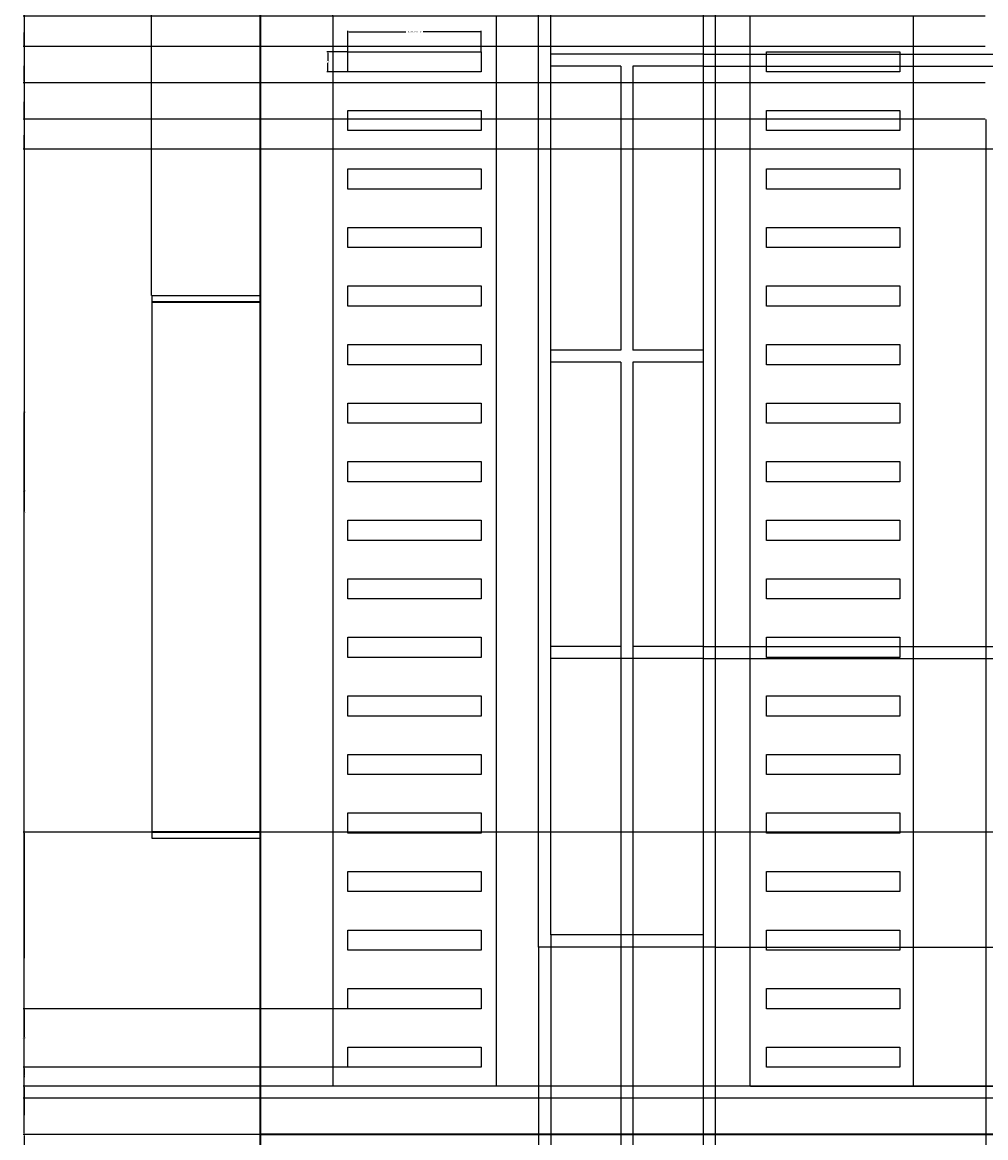
# Model space of a CAD drawing. Units: inches. Extents: x 2148 to 2587, y 1015 to 1466.
# Tile 4 of 7: x 2148 to 2307, y 1166 to 1351. Entities that reach past the tile are written whole.
import ezdxf

# ---------------------------------------------------------------- set-up
doc = ezdxf.new("R2010")
doc.units = ezdxf.units.IN
for name, color, linetype, lineweight in [('A-ANNO-DIMS', 2, 'Continuous', 18), ('A-ELEV', 7, 'Continuous', 35), ('A-GLAZ', 4, 'Continuous', 25)]:
    doc.layers.add(name, color=color, linetype=linetype, lineweight=lineweight)
doc.styles.get("Standard").update_dxf_attribs({"font": 'arial.ttf'})
doc.dimstyles.get("Standard").update_dxf_attribs({"dimtxt": 0.18, "dimasz": 0.18, "dimexe": 0.18, "dimexo": 0.0625, "dimgap": 0.09, "dimtad": 0, "dimtih": 1, "dimtoh": 1, "dimdec": 4, "dimzin": 0, "dimdsep": 46, "dimtxsty": 'Standard', "dimcen": 0.09, "dimadec": 0, "dimazin": 0, "dimtfac": 1, "dimtdec": 4, "dimtofl": 0, "dimtmove": 0, "dimatfit": 3, "dimfxl": 1, "dimtolj": 1, "dimtzin": 0, "dimarcsym": 0})

# ---------------------------------------------------------------- blocks, each defined once
blk = doc.blocks.new('WIN-SIDE')
for p, q in [((18, 89.73), (0, 89.73)), ((18, 0), (18, 89.73)), ((0, 0), (18, 0))]:
    blk.add_line(p, q)
blk = doc.blocks.new('LOUVRE-SLAT')
blk.add_lwpolyline([(2201.49, 1345.86), (2223.57, 1345.86), (2223.57, 1342.52), (2201.49, 1342.52)], close=True)
blk = doc.blocks.new('*D3')
at = {"layer": 'A-ANNO-DIMS', "color": 0, "lineweight": -2, "transparency": 16777216}
for p, q in [((2201.49, 1345.92), (2201.49, 1349.35)), ((2201.67, 1349.17), (2211.11, 1349.17)), ((2223.39, 1349.17), (2213.96, 1349.17)), ((2223.57, 1345.92), (2223.57, 1349.35))]:
    blk.add_line(p, q, dxfattribs=at)
at = {"layer": 'A-ANNO-DIMS', "color": 0, "transparency": 16777216}
for points in [[(2201.67, 1349.2), (2201.67, 1349.14), (2201.49, 1349.17)], [(2223.39, 1349.2), (2223.39, 1349.14), (2223.57, 1349.17)]]:
    blk.add_solid(points, dxfattribs=at)
at = {"layer": 'Defpoints', "color": 0, "transparency": 16777216}
for p in [(2223.57, 1349.17), (2201.49, 1345.86), (2223.57, 1345.86)]:
    blk.add_point(p, dxfattribs=at)
at = {"layer": 'A-ANNO-DIMS', "color": 0, "transparency": 16777216, "insert": (2212.53, 1349.17), "char_height": 0.18, "attachment_point": 5}
blk.add_mtext('\\A1;LOUVRE SLAT 22 TYP.', dxfattribs=at)
blk = doc.blocks.new('*D4')
at = {"layer": 'A-ANNO-DIMS', "color": 0, "lineweight": -2, "transparency": 16777216}
for p, q in [((2201.43, 1345.86), (2198, 1345.86)), ((2198.18, 1345.68), (2198.18, 1344.37)), ((2198.18, 1342.7), (2198.18, 1344.01)), ((2201.43, 1342.52), (2198, 1342.52))]:
    blk.add_line(p, q, dxfattribs=at)
at = {"layer": 'A-ANNO-DIMS', "color": 0, "transparency": 16777216}
for points in [[(2198.15, 1345.68), (2198.21, 1345.68), (2198.18, 1345.86)], [(2198.15, 1342.7), (2198.21, 1342.7), (2198.18, 1342.52)]]:
    blk.add_solid(points, dxfattribs=at)
at = {"layer": 'Defpoints', "color": 0, "transparency": 16777216}
for p in [(2198.18, 1345.86), (2201.49, 1345.86), (2201.49, 1342.52)]:
    blk.add_point(p, dxfattribs=at)
at = {"layer": 'A-ANNO-DIMS', "color": 0, "transparency": 16777216, "insert": (2198.18, 1344.19), "char_height": 0.18, "attachment_point": 5}
blk.add_mtext('\\A1;3 TYP.', dxfattribs=at)
blk = doc.blocks.new('*D7')
at = {"layer": 'A-ANNO-DIMS', "color": 0, "lineweight": -2, "transparency": 16777216}
for p, q in [((2169.03, 1305.54), (2169.03, 1466.02)), ((2169.21, 1465.84), (2175.82, 1465.84)), ((2182.85, 1465.84), (2176.24, 1465.84)), ((2183.03, 1444.81), (2183.03, 1466.02))]:
    blk.add_line(p, q, dxfattribs=at)
at = {"layer": 'A-ANNO-DIMS', "color": 0, "transparency": 16777216}
for points in [[(2169.21, 1465.87), (2169.21, 1465.81), (2169.03, 1465.84)], [(2182.85, 1465.87), (2182.85, 1465.81), (2183.03, 1465.84)]]:
    blk.add_solid(points, dxfattribs=at)
at = {"layer": 'Defpoints', "color": 0, "transparency": 16777216}
for p in [(2183.03, 1465.84), (2183.03, 1444.74), (2169.03, 1305.47)]:
    blk.add_point(p, dxfattribs=at)
at = {"layer": 'A-ANNO-DIMS', "color": 0, "transparency": 16777216, "insert": (2176.03, 1465.84), "char_height": 0.18, "attachment_point": 5}
blk.add_mtext('\\A1;14', dxfattribs=at)
blk = doc.blocks.new('*D22')
at = {"layer": 'A-ANNO-DIMS', "color": 0, "lineweight": -2, "transparency": 16777216}
for p, q in [((2186.971769, 1166.74266), (2147.754269, 1166.74266)), ((2147.934269, 1166.56266), (2147.934269, 1164.92266)), ((2147.934269, 1162.92266), (2147.934269, 1164.56266)), ((2186.971769, 1162.74266), (2147.754269, 1162.74266))]:
    blk.add_line(p, q, dxfattribs=at)
at = {"layer": 'A-ANNO-DIMS', "color": 0, "transparency": 16777216}
for points in [[(2147.904269, 1166.56266), (2147.964269, 1166.56266), (2147.934269, 1166.74266)], [(2147.904269, 1162.92266), (2147.964269, 1162.92266), (2147.934269, 1162.74266)]]:
    blk.add_solid(points, dxfattribs=at)
at = {"layer": 'Defpoints', "color": 0, "transparency": 16777216}
for p in [(2147.934269, 1166.74266), (2187.034269, 1166.74266), (2187.034269, 1162.74266)]:
    blk.add_point(p, dxfattribs=at)
at = {"layer": 'A-ANNO-DIMS', "color": 0, "transparency": 16777216, "insert": (2147.934269, 1164.74266), "char_height": 0.18, "attachment_point": 5}
blk.add_mtext('\\A1;4', dxfattribs=at)
blk = doc.blocks.new('*D23')
at = {"layer": 'A-ANNO-DIMS', "color": 0, "lineweight": -2, "transparency": 16777216}
for p, q in [((2186.97, 1405.74), (2147.75, 1405.74)), ((2147.93, 1405.56), (2147.93, 1286.42)), ((2147.93, 1166.92), (2147.93, 1286.06)), ((2186.97, 1166.74), (2147.75, 1166.74))]:
    blk.add_line(p, q, dxfattribs=at)
at = {"layer": 'A-ANNO-DIMS', "color": 0, "transparency": 16777216}
for points in [[(2147.9, 1405.56), (2147.96, 1405.56), (2147.93, 1405.74)], [(2147.9, 1166.92), (2147.96, 1166.92), (2147.93, 1166.74)]]:
    blk.add_solid(points, dxfattribs=at)
at = {"layer": 'Defpoints', "color": 0, "transparency": 16777216}
for p in [(2147.93, 1405.74), (2187.03, 1405.74), (2187.03, 1166.74)]:
    blk.add_point(p, dxfattribs=at)
at = {"layer": 'A-ANNO-DIMS', "color": 0, "transparency": 16777216, "insert": (2147.93, 1286.24), "char_height": 0.18, "attachment_point": 5}
blk.add_mtext('\\A1;239', dxfattribs=at)
blk = doc.blocks.new('*D47')
at = {"layer": 'A-ANNO-DIMS', "color": 0, "lineweight": -2, "transparency": 16777216}
for p, q in [((2307.03, 1334.68), (2307.03, 1015.46)), ((2316.03, 1329.68), (2316.03, 1015.46)), ((2307.21, 1015.64), (2311.39, 1015.64)), ((2315.85, 1015.64), (2311.68, 1015.64))]:
    blk.add_line(p, q, dxfattribs=at)
at = {"layer": 'A-ANNO-DIMS', "color": 0, "transparency": 16777216}
for points in [[(2307.21, 1015.67), (2307.21, 1015.61), (2307.03, 1015.64)], [(2315.85, 1015.67), (2315.85, 1015.61), (2316.03, 1015.64)]]:
    blk.add_solid(points, dxfattribs=at)
at = {"layer": 'Defpoints', "color": 0, "transparency": 16777216}
for p in [(2307.03, 1334.74), (2316.03, 1329.74), (2316.03, 1015.64)]:
    blk.add_point(p, dxfattribs=at)
at = {"layer": 'A-ANNO-DIMS', "color": 0, "transparency": 16777216, "insert": (2311.53, 1015.64), "char_height": 0.18, "attachment_point": 5}
blk.add_mtext('\\A1;9', dxfattribs=at)
blk = doc.blocks.new('*D58')
at = {"layer": 'A-ANNO-DIMS', "color": 0, "lineweight": -2, "transparency": 16777216}
for p, q in [((2306.971769, 1166.74266), (2147.754269, 1166.74266)), ((2147.934269, 1166.56266), (2147.934269, 1164.92266)), ((2147.934269, 1162.92266), (2147.934269, 1164.56266)), ((2306.971769, 1162.74266), (2147.754269, 1162.74266))]:
    blk.add_line(p, q, dxfattribs=at)
at = {"layer": 'A-ANNO-DIMS', "color": 0, "transparency": 16777216}
for points in [[(2147.904269, 1166.56266), (2147.964269, 1166.56266), (2147.934269, 1166.74266)], [(2147.904269, 1162.92266), (2147.964269, 1162.92266), (2147.934269, 1162.74266)]]:
    blk.add_solid(points, dxfattribs=at)
at = {"layer": 'Defpoints', "color": 0, "transparency": 16777216}
for p in [(2147.934269, 1166.74266), (2307.034269, 1166.74266), (2307.034269, 1162.74266)]:
    blk.add_point(p, dxfattribs=at)
at = {"layer": 'A-ANNO-DIMS', "color": 0, "transparency": 16777216, "insert": (2147.934269, 1164.74266), "char_height": 0.18, "attachment_point": 5}
blk.add_mtext('\\A1;4', dxfattribs=at)
blk = doc.blocks.new('*D59')
at = {"layer": 'A-ANNO-DIMS', "color": 0, "lineweight": -2, "transparency": 16777216}
for p, q in [((2315.97, 1172.74), (2147.75, 1172.74)), ((2147.93, 1172.56), (2147.93, 1169.92)), ((2147.93, 1166.92), (2147.93, 1169.56)), ((2306.97, 1166.74), (2147.75, 1166.74))]:
    blk.add_line(p, q, dxfattribs=at)
at = {"layer": 'A-ANNO-DIMS', "color": 0, "transparency": 16777216}
for points in [[(2147.9, 1172.56), (2147.96, 1172.56), (2147.93, 1172.74)], [(2147.9, 1166.92), (2147.96, 1166.92), (2147.93, 1166.74)]]:
    blk.add_solid(points, dxfattribs=at)
at = {"layer": 'Defpoints', "color": 0, "transparency": 16777216}
for p in [(2147.93, 1172.74), (2316.03, 1172.74), (2307.03, 1166.74)]:
    blk.add_point(p, dxfattribs=at)
at = {"layer": 'A-ANNO-DIMS', "color": 0, "transparency": 16777216, "insert": (2147.93, 1169.74), "char_height": 0.18, "attachment_point": 5}
blk.add_mtext('\\A1;6', dxfattribs=at)
blk = doc.blocks.new('*D60')
at = {"layer": 'A-ANNO-DIMS', "color": 0, "lineweight": -2, "transparency": 16777216}
for p, q in [((2315.97, 1174.74), (2147.75, 1174.74)), ((2147.93, 1174.56), (2147.93, 1173.92)), ((2315.97, 1172.74), (2147.75, 1172.74)), ((2147.93, 1172.92), (2147.93, 1173.56))]:
    blk.add_line(p, q, dxfattribs=at)
at = {"layer": 'A-ANNO-DIMS', "color": 0, "transparency": 16777216}
for points in [[(2147.9, 1174.56), (2147.96, 1174.56), (2147.93, 1174.74)], [(2147.9, 1172.92), (2147.96, 1172.92), (2147.93, 1172.74)]]:
    blk.add_solid(points, dxfattribs=at)
at = {"layer": 'Defpoints', "color": 0, "transparency": 16777216}
for p in [(2147.93, 1174.74), (2316.03, 1174.74), (2316.03, 1172.74)]:
    blk.add_point(p, dxfattribs=at)
at = {"layer": 'A-ANNO-DIMS', "color": 0, "transparency": 16777216, "insert": (2147.93, 1173.74), "char_height": 0.18, "attachment_point": 5}
blk.add_mtext('\\A1;2', dxfattribs=at)
blk = doc.blocks.new('*D61')
at = {"layer": 'A-ANNO-DIMS', "color": 0, "lineweight": -2, "transparency": 16777216}
for p, q in [((2315.97, 1216.74), (2147.75, 1216.74)), ((2147.93, 1216.56), (2147.93, 1195.92)), ((2147.93, 1174.92), (2147.93, 1195.56)), ((2315.97, 1174.74), (2147.75, 1174.74))]:
    blk.add_line(p, q, dxfattribs=at)
at = {"layer": 'A-ANNO-DIMS', "color": 0, "transparency": 16777216}
for points in [[(2147.9, 1216.56), (2147.96, 1216.56), (2147.93, 1216.74)], [(2147.9, 1174.92), (2147.96, 1174.92), (2147.93, 1174.74)]]:
    blk.add_solid(points, dxfattribs=at)
at = {"layer": 'Defpoints', "color": 0, "transparency": 16777216}
for p in [(2147.93, 1216.74), (2316.03, 1216.74), (2316.03, 1174.74)]:
    blk.add_point(p, dxfattribs=at)
at = {"layer": 'A-ANNO-DIMS', "color": 0, "transparency": 16777216, "insert": (2147.93, 1195.74), "char_height": 0.18, "attachment_point": 5}
blk.add_mtext('\\A1;42', dxfattribs=at)
blk = doc.blocks.new('*D62')
at = {"layer": 'A-ANNO-DIMS', "color": 0, "lineweight": -2, "transparency": 16777216}
for p, q in [((2315.97, 1329.74), (2147.75, 1329.74)), ((2147.93, 1329.56), (2147.93, 1273.42)), ((2147.93, 1216.92), (2147.93, 1273.06)), ((2315.97, 1216.74), (2147.75, 1216.74))]:
    blk.add_line(p, q, dxfattribs=at)
at = {"layer": 'A-ANNO-DIMS', "color": 0, "transparency": 16777216}
for points in [[(2147.9, 1329.56), (2147.96, 1329.56), (2147.93, 1329.74)], [(2147.9, 1216.92), (2147.96, 1216.92), (2147.93, 1216.74)]]:
    blk.add_solid(points, dxfattribs=at)
at = {"layer": 'Defpoints', "color": 0, "transparency": 16777216}
for p in [(2147.93, 1329.74), (2316.03, 1329.74), (2316.03, 1216.74)]:
    blk.add_point(p, dxfattribs=at)
at = {"layer": 'A-ANNO-DIMS', "color": 0, "transparency": 16777216, "insert": (2147.93, 1273.24), "char_height": 0.18, "attachment_point": 5}
blk.add_mtext('\\A1;113', dxfattribs=at)
blk = doc.blocks.new('*D63')
at = {"layer": 'A-ANNO-DIMS', "color": 0, "lineweight": -2, "transparency": 16777216}
for p, q in [((2306.97, 1334.74), (2147.75, 1334.74)), ((2147.93, 1334.56), (2147.93, 1332.42)), ((2147.93, 1329.92), (2147.93, 1332.06)), ((2315.97, 1329.74), (2147.75, 1329.74))]:
    blk.add_line(p, q, dxfattribs=at)
at = {"layer": 'A-ANNO-DIMS', "color": 0, "transparency": 16777216}
for points in [[(2147.9, 1334.56), (2147.96, 1334.56), (2147.93, 1334.74)], [(2147.9, 1329.92), (2147.96, 1329.92), (2147.93, 1329.74)]]:
    blk.add_solid(points, dxfattribs=at)
at = {"layer": 'Defpoints', "color": 0, "transparency": 16777216}
for p in [(2147.93, 1334.74), (2307.03, 1334.74), (2316.03, 1329.74)]:
    blk.add_point(p, dxfattribs=at)
at = {"layer": 'A-ANNO-DIMS', "color": 0, "transparency": 16777216, "insert": (2147.93, 1332.24), "char_height": 0.18, "attachment_point": 5}
blk.add_mtext('\\A1;5', dxfattribs=at)
blk = doc.blocks.new('*D64')
at = {"layer": 'A-ANNO-DIMS', "color": 0, "lineweight": -2, "transparency": 16777216}
for p, q in [((2306.97, 1340.74), (2147.75, 1340.74)), ((2147.93, 1340.56), (2147.93, 1337.92)), ((2147.93, 1334.92), (2147.93, 1337.56)), ((2306.97, 1334.74), (2147.75, 1334.74))]:
    blk.add_line(p, q, dxfattribs=at)
at = {"layer": 'A-ANNO-DIMS', "color": 0, "transparency": 16777216}
for points in [[(2147.9, 1340.56), (2147.96, 1340.56), (2147.93, 1340.74)], [(2147.9, 1334.92), (2147.96, 1334.92), (2147.93, 1334.74)]]:
    blk.add_solid(points, dxfattribs=at)
at = {"layer": 'Defpoints', "color": 0, "transparency": 16777216}
for p in [(2147.93, 1340.74), (2307.03, 1340.74), (2307.03, 1334.74)]:
    blk.add_point(p, dxfattribs=at)
at = {"layer": 'A-ANNO-DIMS', "color": 0, "transparency": 16777216, "insert": (2147.93, 1337.74), "char_height": 0.18, "attachment_point": 5}
blk.add_mtext('\\A1;6', dxfattribs=at)
blk = doc.blocks.new('*D65')
at = {"layer": 'A-ANNO-DIMS', "color": 0, "lineweight": -2, "transparency": 16777216}
for p, q in [((2306.97, 1346.74), (2147.75, 1346.74)), ((2147.93, 1346.56), (2147.93, 1343.92)), ((2147.93, 1340.92), (2147.93, 1343.56)), ((2306.97, 1340.74), (2147.75, 1340.74))]:
    blk.add_line(p, q, dxfattribs=at)
at = {"layer": 'A-ANNO-DIMS', "color": 0, "transparency": 16777216}
for points in [[(2147.9, 1346.56), (2147.96, 1346.56), (2147.93, 1346.74)], [(2147.9, 1340.92), (2147.96, 1340.92), (2147.93, 1340.74)]]:
    blk.add_solid(points, dxfattribs=at)
at = {"layer": 'Defpoints', "color": 0, "transparency": 16777216}
for p in [(2147.93, 1346.74), (2307.03, 1346.74), (2307.03, 1340.74)]:
    blk.add_point(p, dxfattribs=at)
at = {"layer": 'A-ANNO-DIMS', "color": 0, "transparency": 16777216, "insert": (2147.93, 1343.74), "char_height": 0.18, "attachment_point": 5}
blk.add_mtext('\\A1;6', dxfattribs=at)
blk = doc.blocks.new('*D66')
at = {"layer": 'A-ANNO-DIMS', "color": 0, "lineweight": -2, "transparency": 16777216}
for p, q in [((2306.97, 1351.74), (2147.75, 1351.74)), ((2147.93, 1351.56), (2147.93, 1349.42)), ((2147.93, 1346.92), (2147.93, 1349.06)), ((2306.97, 1346.74), (2147.75, 1346.74))]:
    blk.add_line(p, q, dxfattribs=at)
at = {"layer": 'A-ANNO-DIMS', "color": 0, "transparency": 16777216}
for points in [[(2147.9, 1351.56), (2147.96, 1351.56), (2147.93, 1351.74)], [(2147.9, 1346.92), (2147.96, 1346.92), (2147.93, 1346.74)]]:
    blk.add_solid(points, dxfattribs=at)
at = {"layer": 'Defpoints', "color": 0, "transparency": 16777216}
for p in [(2147.93, 1351.74), (2307.03, 1351.74), (2307.03, 1346.74)]:
    blk.add_point(p, dxfattribs=at)
at = {"layer": 'A-ANNO-DIMS', "color": 0, "transparency": 16777216, "insert": (2147.93, 1349.24), "char_height": 0.18, "attachment_point": 5}
blk.add_mtext('\\A1;5', dxfattribs=at)
blk = doc.blocks.new('*D73')
at = {"layer": 'A-ANNO-DIMS', "color": 0, "lineweight": -2, "transparency": 16777216}
for p, q in [((2187.03, 1166.81), (2187.03, 1466.02)), ((2187.21, 1465.84), (2192.82, 1465.84)), ((2198.85, 1465.84), (2193.24, 1465.84)), ((2199.03, 1351.81), (2199.03, 1466.02))]:
    blk.add_line(p, q, dxfattribs=at)
at = {"layer": 'A-ANNO-DIMS', "color": 0, "transparency": 16777216}
for points in [[(2187.21, 1465.87), (2187.21, 1465.81), (2187.03, 1465.84)], [(2198.85, 1465.87), (2198.85, 1465.81), (2199.03, 1465.84)]]:
    blk.add_solid(points, dxfattribs=at)
at = {"layer": 'Defpoints', "color": 0, "transparency": 16777216}
for p in [(2199.03, 1465.84), (2199.03, 1351.74), (2187.03, 1166.74)]:
    blk.add_point(p, dxfattribs=at)
at = {"layer": 'A-ANNO-DIMS', "color": 0, "transparency": 16777216, "insert": (2193.03, 1465.84), "char_height": 0.18, "attachment_point": 5}
blk.add_mtext('\\A1;12', dxfattribs=at)
blk = doc.blocks.new('*D83')
at = {"layer": 'A-ANNO-DIMS', "color": 0, "lineweight": -2, "transparency": 16777216}
for p, q in [((2235.06, 1199.68), (2235.06, 1015.46)), ((2233.06, 1197.68), (2233.06, 1015.46)), ((2233.24, 1015.64), (2233.91, 1015.64)), ((2234.88, 1015.64), (2234.21, 1015.64))]:
    blk.add_line(p, q, dxfattribs=at)
at = {"layer": 'A-ANNO-DIMS', "color": 0, "transparency": 16777216}
for points in [[(2233.24, 1015.67), (2233.24, 1015.61), (2233.06, 1015.64)], [(2234.88, 1015.67), (2234.88, 1015.61), (2235.06, 1015.64)]]:
    blk.add_solid(points, dxfattribs=at)
at = {"layer": 'Defpoints', "color": 0, "transparency": 16777216}
for p in [(2235.06, 1199.74), (2233.06, 1197.74), (2235.06, 1015.64)]:
    blk.add_point(p, dxfattribs=at)
at = {"layer": 'A-ANNO-DIMS', "color": 0, "transparency": 16777216, "insert": (2234.06, 1015.64), "char_height": 0.18, "attachment_point": 5}
blk.add_mtext('\\A1;2', dxfattribs=at)
blk = doc.blocks.new('*D84')
at = {"layer": 'A-ANNO-DIMS', "color": 0, "lineweight": -2, "transparency": 16777216}
for p, q in [((2246.67, 1247.43), (2246.67, 1015.46)), ((2235.06, 1199.68), (2235.06, 1015.46)), ((2235.24, 1015.64), (2240.41, 1015.64)), ((2246.49, 1015.64), (2241.32, 1015.64))]:
    blk.add_line(p, q, dxfattribs=at)
at = {"layer": 'A-ANNO-DIMS', "color": 0, "transparency": 16777216}
for points in [[(2235.24, 1015.67), (2235.24, 1015.61), (2235.06, 1015.64)], [(2246.49, 1015.67), (2246.49, 1015.61), (2246.67, 1015.64)]]:
    blk.add_solid(points, dxfattribs=at)
at = {"layer": 'Defpoints', "color": 0, "transparency": 16777216}
for p in [(2246.67, 1247.49), (2235.06, 1199.74), (2246.67, 1015.64)]:
    blk.add_point(p, dxfattribs=at)
at = {"layer": 'A-ANNO-DIMS', "color": 0, "transparency": 16777216, "insert": (2240.87, 1015.64), "char_height": 0.18, "attachment_point": 5}
blk.add_mtext('\\A1;11.613', dxfattribs=at)
blk = doc.blocks.new('*D85')
at = {"layer": 'A-ANNO-DIMS', "color": 0, "lineweight": -2, "transparency": 16777216}
for p, q in [((2246.67, 1247.43), (2246.67, 1015.46)), ((2248.67, 1247.43), (2248.67, 1015.46)), ((2246.85, 1015.64), (2247.52, 1015.64)), ((2248.49, 1015.64), (2247.82, 1015.64))]:
    blk.add_line(p, q, dxfattribs=at)
at = {"layer": 'A-ANNO-DIMS', "color": 0, "transparency": 16777216}
for points in [[(2246.85, 1015.67), (2246.85, 1015.61), (2246.67, 1015.64)], [(2248.49, 1015.67), (2248.49, 1015.61), (2248.67, 1015.64)]]:
    blk.add_solid(points, dxfattribs=at)
at = {"layer": 'Defpoints', "color": 0, "transparency": 16777216}
for p in [(2246.67, 1247.49), (2248.67, 1247.49), (2248.67, 1015.64)]:
    blk.add_point(p, dxfattribs=at)
at = {"layer": 'A-ANNO-DIMS', "color": 0, "transparency": 16777216, "insert": (2247.67, 1015.64), "char_height": 0.18, "attachment_point": 5}
blk.add_mtext('\\A1;2', dxfattribs=at)
blk = doc.blocks.new('*D86')
at = {"layer": 'A-ANNO-DIMS', "color": 0, "lineweight": -2, "transparency": 16777216}
for p, q in [((2248.67, 1247.43), (2248.67, 1015.46)), ((2260.29, 1199.68), (2260.29, 1015.46)), ((2248.85, 1015.64), (2254.03, 1015.64)), ((2260.11, 1015.64), (2254.94, 1015.64))]:
    blk.add_line(p, q, dxfattribs=at)
at = {"layer": 'A-ANNO-DIMS', "color": 0, "transparency": 16777216}
for points in [[(2248.85, 1015.67), (2248.85, 1015.61), (2248.67, 1015.64)], [(2260.11, 1015.67), (2260.11, 1015.61), (2260.29, 1015.64)]]:
    blk.add_solid(points, dxfattribs=at)
at = {"layer": 'Defpoints', "color": 0, "transparency": 16777216}
for p in [(2248.67, 1247.49), (2260.29, 1199.74), (2260.29, 1015.64)]:
    blk.add_point(p, dxfattribs=at)
at = {"layer": 'A-ANNO-DIMS', "color": 0, "transparency": 16777216, "insert": (2254.48, 1015.64), "char_height": 0.18, "attachment_point": 5}
blk.add_mtext('\\A1;11.613', dxfattribs=at)
blk = doc.blocks.new('*D87')
at = {"layer": 'A-ANNO-DIMS', "color": 0, "lineweight": -2, "transparency": 16777216}
for p, q in [((2260.29, 1199.68), (2260.29, 1015.46)), ((2262.29, 1197.68), (2262.29, 1015.46)), ((2260.47, 1015.64), (2261.14, 1015.64)), ((2262.11, 1015.64), (2261.44, 1015.64))]:
    blk.add_line(p, q, dxfattribs=at)
at = {"layer": 'A-ANNO-DIMS', "color": 0, "transparency": 16777216}
for points in [[(2260.47, 1015.67), (2260.47, 1015.61), (2260.29, 1015.64)], [(2262.11, 1015.67), (2262.11, 1015.61), (2262.29, 1015.64)]]:
    blk.add_solid(points, dxfattribs=at)
at = {"layer": 'Defpoints', "color": 0, "transparency": 16777216}
for p in [(2260.29, 1199.74), (2262.29, 1197.74), (2262.29, 1015.64)]:
    blk.add_point(p, dxfattribs=at)
at = {"layer": 'A-ANNO-DIMS', "color": 0, "transparency": 16777216, "insert": (2261.29, 1015.64), "char_height": 0.18, "attachment_point": 5}
blk.add_mtext('\\A1;2', dxfattribs=at)
blk = doc.blocks.new('*D88')
at = {"layer": 'A-ANNO-DIMS', "color": 0, "lineweight": -2, "transparency": 16777216}
for p, q in [((2198.97, 1174.74), (2147.75, 1174.74)), ((2147.93, 1174.56), (2147.93, 1170.92)), ((2147.93, 1166.92), (2147.93, 1170.56)), ((2186.97, 1166.74), (2147.75, 1166.74))]:
    blk.add_line(p, q, dxfattribs=at)
at = {"layer": 'A-ANNO-DIMS', "color": 0, "transparency": 16777216}
for points in [[(2147.9, 1174.56), (2147.96, 1174.56), (2147.93, 1174.74)], [(2147.9, 1166.92), (2147.96, 1166.92), (2147.93, 1166.74)]]:
    blk.add_solid(points, dxfattribs=at)
at = {"layer": 'Defpoints', "color": 0, "transparency": 16777216}
for p in [(2147.93, 1174.74), (2199.03, 1174.74), (2187.03, 1166.74)]:
    blk.add_point(p, dxfattribs=at)
at = {"layer": 'A-ANNO-DIMS', "color": 0, "transparency": 16777216, "insert": (2147.93, 1170.74), "char_height": 0.18, "attachment_point": 5}
blk.add_mtext('\\A1;8', dxfattribs=at)
blk = doc.blocks.new('*D89')
at = {"layer": 'A-ANNO-DIMS', "color": 0, "lineweight": -2, "transparency": 16777216}
for p, q in [((2201.43, 1177.84), (2147.75, 1177.84)), ((2147.93, 1177.66), (2147.93, 1176.47)), ((2147.93, 1174.92), (2147.93, 1176.11)), ((2198.97, 1174.74), (2147.75, 1174.74))]:
    blk.add_line(p, q, dxfattribs=at)
at = {"layer": 'A-ANNO-DIMS', "color": 0, "transparency": 16777216}
for points in [[(2147.9, 1177.66), (2147.96, 1177.66), (2147.93, 1177.84)], [(2147.9, 1174.92), (2147.96, 1174.92), (2147.93, 1174.74)]]:
    blk.add_solid(points, dxfattribs=at)
at = {"layer": 'Defpoints', "color": 0, "transparency": 16777216}
for p in [(2147.93, 1177.84), (2201.49, 1177.84), (2199.03, 1174.74)]:
    blk.add_point(p, dxfattribs=at)
at = {"layer": 'A-ANNO-DIMS', "color": 0, "transparency": 16777216, "insert": (2147.93, 1176.29), "char_height": 0.18, "attachment_point": 5}
blk.add_mtext('\\A1;3.1', dxfattribs=at)
blk = doc.blocks.new('*D90')
at = {"layer": 'A-ANNO-DIMS', "color": 0, "lineweight": -2, "transparency": 16777216}
for p, q in [((2201.43, 1187.53), (2147.75, 1187.53)), ((2147.93, 1187.35), (2147.93, 1182.87)), ((2147.93, 1178.02), (2147.93, 1182.5)), ((2201.43, 1177.84), (2147.75, 1177.84))]:
    blk.add_line(p, q, dxfattribs=at)
at = {"layer": 'A-ANNO-DIMS', "color": 0, "transparency": 16777216}
for points in [[(2147.9, 1187.35), (2147.96, 1187.35), (2147.93, 1187.53)], [(2147.9, 1178.02), (2147.96, 1178.02), (2147.93, 1177.84)]]:
    blk.add_solid(points, dxfattribs=at)
at = {"layer": 'Defpoints', "color": 0, "transparency": 16777216}
for p in [(2147.93, 1187.53), (2201.49, 1187.53), (2201.49, 1177.84)]:
    blk.add_point(p, dxfattribs=at)
at = {"layer": 'A-ANNO-DIMS', "color": 0, "transparency": 16777216, "insert": (2147.93, 1182.69), "char_height": 0.18, "attachment_point": 5}
blk.add_mtext('\\A1;9.687', dxfattribs=at)
blk = doc.blocks.new('*D91')
at = {"layer": 'A-ANNO-DIMS', "color": 0, "lineweight": -2, "transparency": 16777216}
for p, q in [((2198.97, 1351.74), (2147.75, 1351.74)), ((2147.93, 1351.56), (2147.93, 1269.82)), ((2147.93, 1187.71), (2147.93, 1269.45)), ((2201.43, 1187.53), (2147.75, 1187.53))]:
    blk.add_line(p, q, dxfattribs=at)
at = {"layer": 'A-ANNO-DIMS', "color": 0, "transparency": 16777216}
for points in [[(2147.9, 1351.56), (2147.96, 1351.56), (2147.93, 1351.74)], [(2147.9, 1187.71), (2147.96, 1187.71), (2147.93, 1187.53)]]:
    blk.add_solid(points, dxfattribs=at)
at = {"layer": 'Defpoints', "color": 0, "transparency": 16777216}
for p in [(2147.93, 1351.74), (2199.03, 1351.74), (2201.49, 1187.53)]:
    blk.add_point(p, dxfattribs=at)
at = {"layer": 'A-ANNO-DIMS', "color": 0, "transparency": 16777216, "insert": (2147.93, 1269.64), "char_height": 0.18, "attachment_point": 5}
blk.add_mtext('\\A1;164.2', dxfattribs=at)
blk = doc.blocks.new('*D92')
at = {"layer": 'A-ANNO-DIMS', "color": 0, "lineweight": -2, "transparency": 16777216}
for p, q in [((2262.35, 1197.74), (2586.31, 1197.74)), ((2586.13, 1197.56), (2586.13, 1186.42)), ((2586.13, 1174.92), (2586.13, 1186.06)), ((2268.1, 1174.74), (2586.31, 1174.74))]:
    blk.add_line(p, q, dxfattribs=at)
at = {"layer": 'A-ANNO-DIMS', "color": 0, "transparency": 16777216}
for points in [[(2586.1, 1197.56), (2586.16, 1197.56), (2586.13, 1197.74)], [(2586.1, 1174.92), (2586.16, 1174.92), (2586.13, 1174.74)]]:
    blk.add_solid(points, dxfattribs=at)
at = {"layer": 'Defpoints', "color": 0, "transparency": 16777216}
for p in [(2262.29, 1197.74), (2586.13, 1197.74), (2268.03, 1174.74)]:
    blk.add_point(p, dxfattribs=at)
at = {"layer": 'A-ANNO-DIMS', "color": 0, "transparency": 16777216, "insert": (2586.13, 1186.24), "char_height": 0.18, "attachment_point": 5}
blk.add_mtext('\\A1;22.995', dxfattribs=at)
blk = doc.blocks.new('*D93')
at = {"layer": 'A-ANNO-DIMS', "color": 0, "lineweight": -2, "transparency": 16777216}
for p, q in [((2260.35, 1245.49), (2586.31, 1245.49)), ((2586.13, 1245.31), (2586.13, 1221.79)), ((2586.13, 1197.92), (2586.13, 1221.43)), ((2262.35, 1197.74), (2586.31, 1197.74))]:
    blk.add_line(p, q, dxfattribs=at)
at = {"layer": 'A-ANNO-DIMS', "color": 0, "transparency": 16777216}
for points in [[(2586.1, 1245.31), (2586.16, 1245.31), (2586.13, 1245.49)], [(2586.1, 1197.92), (2586.16, 1197.92), (2586.13, 1197.74)]]:
    blk.add_solid(points, dxfattribs=at)
at = {"layer": 'Defpoints', "color": 0, "transparency": 16777216}
for p in [(2260.29, 1245.49), (2586.13, 1245.49), (2262.29, 1197.74)]:
    blk.add_point(p, dxfattribs=at)
at = {"layer": 'A-ANNO-DIMS', "color": 0, "transparency": 16777216, "insert": (2586.13, 1221.61), "char_height": 0.18, "attachment_point": 5}
blk.add_mtext('\\A1;47.75', dxfattribs=at)
blk = doc.blocks.new('*D94')
at = {"layer": 'A-ANNO-DIMS', "color": 0, "lineweight": -2, "transparency": 16777216}
for p, q in [((2260.35, 1247.49), (2586.31, 1247.49)), ((2586.13, 1247.31), (2586.13, 1246.67)), ((2586.13, 1245.67), (2586.13, 1246.31)), ((2260.35, 1245.49), (2586.31, 1245.49))]:
    blk.add_line(p, q, dxfattribs=at)
at = {"layer": 'A-ANNO-DIMS', "color": 0, "transparency": 16777216}
for points in [[(2586.1, 1247.31), (2586.16, 1247.31), (2586.13, 1247.49)], [(2586.1, 1245.67), (2586.16, 1245.67), (2586.13, 1245.49)]]:
    blk.add_solid(points, dxfattribs=at)
at = {"layer": 'Defpoints', "color": 0, "transparency": 16777216}
for p in [(2260.29, 1247.49), (2586.13, 1247.49), (2260.29, 1245.49)]:
    blk.add_point(p, dxfattribs=at)
at = {"layer": 'A-ANNO-DIMS', "color": 0, "transparency": 16777216, "insert": (2586.13, 1246.49), "char_height": 0.18, "attachment_point": 5}
blk.add_mtext('\\A1;2', dxfattribs=at)
blk = doc.blocks.new('*D95')
at = {"layer": 'A-ANNO-DIMS', "color": 0, "lineweight": -2, "transparency": 16777216}
for p, q in [((2260.35, 1343.49), (2586.31, 1343.49)), ((2586.13, 1343.31), (2586.13, 1295.67)), ((2586.13, 1247.67), (2586.13, 1295.31)), ((2260.35, 1247.49), (2586.31, 1247.49))]:
    blk.add_line(p, q, dxfattribs=at)
at = {"layer": 'A-ANNO-DIMS', "color": 0, "transparency": 16777216}
for points in [[(2586.1, 1343.31), (2586.16, 1343.31), (2586.13, 1343.49)], [(2586.1, 1247.67), (2586.16, 1247.67), (2586.13, 1247.49)]]:
    blk.add_solid(points, dxfattribs=at)
at = {"layer": 'Defpoints', "color": 0, "transparency": 16777216}
for p in [(2260.29, 1343.49), (2586.13, 1343.49), (2260.29, 1247.49)]:
    blk.add_point(p, dxfattribs=at)
at = {"layer": 'A-ANNO-DIMS', "color": 0, "transparency": 16777216, "insert": (2586.13, 1295.49), "char_height": 0.18, "attachment_point": 5}
blk.add_mtext('\\A1;96', dxfattribs=at)
blk = doc.blocks.new('*D96')
at = {"layer": 'A-ANNO-DIMS', "color": 0, "lineweight": -2, "transparency": 16777216}
for p, q in [((2260.35, 1345.49), (2586.31, 1345.49)), ((2586.13, 1345.31), (2586.13, 1344.67)), ((2586.13, 1343.67), (2586.13, 1344.31)), ((2260.35, 1343.49), (2586.31, 1343.49))]:
    blk.add_line(p, q, dxfattribs=at)
at = {"layer": 'A-ANNO-DIMS', "color": 0, "transparency": 16777216}
for points in [[(2586.1, 1345.31), (2586.16, 1345.31), (2586.13, 1345.49)], [(2586.1, 1343.67), (2586.16, 1343.67), (2586.13, 1343.49)]]:
    blk.add_solid(points, dxfattribs=at)
at = {"layer": 'Defpoints', "color": 0, "transparency": 16777216}
for p in [(2260.29, 1345.49), (2586.13, 1345.49), (2260.29, 1343.49)]:
    blk.add_point(p, dxfattribs=at)
at = {"layer": 'A-ANNO-DIMS', "color": 0, "transparency": 16777216, "insert": (2586.13, 1344.49), "char_height": 0.18, "attachment_point": 5}
blk.add_mtext('\\A1;2', dxfattribs=at)
blk = doc.blocks.new('*D97')
at = {"layer": 'A-ANNO-DIMS', "color": 0, "lineweight": -2, "transparency": 16777216}
for p, q in [((2262.35, 1393.24), (2586.31, 1393.24)), ((2586.13, 1393.06), (2586.13, 1369.55)), ((2586.13, 1345.67), (2586.13, 1369.18)), ((2260.35, 1345.49), (2586.31, 1345.49))]:
    blk.add_line(p, q, dxfattribs=at)
at = {"layer": 'A-ANNO-DIMS', "color": 0, "transparency": 16777216}
for points in [[(2586.1, 1393.06), (2586.16, 1393.06), (2586.13, 1393.24)], [(2586.1, 1345.67), (2586.16, 1345.67), (2586.13, 1345.49)]]:
    blk.add_solid(points, dxfattribs=at)
at = {"layer": 'Defpoints', "color": 0, "transparency": 16777216}
for p in [(2262.29, 1393.24), (2586.13, 1393.24), (2260.29, 1345.49)]:
    blk.add_point(p, dxfattribs=at)
at = {"layer": 'A-ANNO-DIMS', "color": 0, "transparency": 16777216, "insert": (2586.13, 1369.36), "char_height": 0.18, "attachment_point": 5}
blk.add_mtext('\\A1;47.75', dxfattribs=at)

msp = doc.modelspace()

# ---------------------------------------------------------------- linework, layer by layer
at = {"layer": 'A-ELEV'}
for p, q in [((2187.0343, 1048.7427), (2187.0343, 1438.7427)), ((2169.0343, 1304.4734), (2187.0343, 1304.4734)), ((2187.0343, 1216.7427), (2169.0343, 1216.7427)), ((2547.0343, 1166.7427), (2187.0343, 1166.7427))]:
    msp.add_line(p, q, dxfattribs=at)
at = {"layer": 'A-GLAZ'}
for p, q in [((2199.0343, 1351.7427), (2199.0343, 1174.7427)), ((2226.0343, 1351.7427), (2226.0343, 1174.7427)), ((2268.0343, 1351.7427), (2268.0343, 1174.7427)), ((2295.0343, 1351.7427), (2295.0343, 1174.7427)), ((2260.287, 1345.4885), (2235.0602, 1345.4885)), ((2246.6736, 1343.4885), (2235.0602, 1343.4885)), ((2246.6736, 1343.4885), (2246.6736, 1296.4885)), ((2260.287, 1343.4885), (2248.6736, 1343.4885)), ((2248.6736, 1343.4885), (2248.6736, 1296.4885)), ((2246.6736, 1296.4885), (2235.0602, 1296.4885)), ((2260.287, 1296.4885), (2248.6736, 1296.4885)), ((2246.6736, 1294.4885), (2235.0602, 1294.4885)), ((2246.6736, 1294.4885), (2246.6736, 1247.4885)), ((2260.287, 1294.4885), (2248.6736, 1294.4885)), ((2248.6736, 1294.4885), (2248.6736, 1247.4885)), ((2246.6736, 1247.4885), (2235.0602, 1247.4885)), ((2260.287, 1247.4885), (2248.6736, 1247.4885)), ((2260.287, 1245.4885), (2235.0602, 1245.4885)), ((2226.0343, 1174.7427), (2199.0343, 1174.7427)), ((2295.0343, 1174.7427), (2268.0343, 1174.7427))]:
    msp.add_line(p, q, dxfattribs=at)
for points in [[(2262.287, 1197.738), (2233.0602, 1197.738), (2233.0602, 1393.2389), (2262.287, 1393.2389)], [(2260.287, 1199.738), (2235.0602, 1199.738), (2235.0602, 1391.2389), (2260.287, 1391.2389)]]:
    msp.add_lwpolyline(points, close=True, dxfattribs=at)

# ---------------------------------------------------------------- block references
for p in [(0, 0), (69.2498, 0), (0, -9.6867), (69.2498, -9.6867), (0, -19.3735), (69.2498, -19.3735), (0, -29.0602), (69.2498, -29.0602), (0, -38.747), (69.2498, -38.747), (0, -48.4337), (69.2498, -48.4337), (0, -58.1205), (69.2498, -58.1205), (0, -67.8072), (69.2498, -67.8072), (0, -77.494), (69.2498, -77.494), (0, -87.1807), (69.2498, -87.1807), (0, -96.8675), (69.2498, -96.8675), (0, -106.5542), (69.2498, -106.5542), (0, -116.241), (69.2498, -116.241), (0, -125.9277), (69.2498, -125.9277), (0, -135.6145), (69.2498, -135.6145), (0, -145.3012), (69.2498, -145.3012), (0, -154.988), (69.2498, -154.988), (0, -164.6747), (69.2498, -164.6747)]:
    msp.add_blockref('LOUVRE-SLAT', p, dxfattribs=at)
at = {"layer": 'A-GLAZ', "rotation": 180}
msp.add_blockref('WIN-SIDE', (2187.0345, 1305.4731), dxfattribs=at)

# ---------------------------------------------------------------- dimensions: what is measured, and where the dimension line sits
at = {"layer": 'A-ANNO-DIMS'}
for base, p1, p2, override, picture, middle in [((2183.0343, 1465.8427), (2169.0343, 1305.4734), (2183.0343, 1444.7427), {"dimdec": 0, "dimlfac": 1, "dimrnd": 0, "dimzin": 0, "dimdsep": 46, "dimlunit": 2}, '*D7', (2176.0343, 1465.8427)), ((2199.0343, 1465.8427), (2187.0343, 1166.7427), (2199.0343, 1351.7427), {"dimdec": 0, "dimlfac": 1, "dimrnd": 0, "dimzin": 0, "dimdsep": 46, "dimlunit": 2}, '*D73', (2193.0343, 1465.8427)), ((2316.0343, 1015.6427), (2307.0343, 1334.7427), (2316.0343, 1329.7427), {"dimdec": 0, "dimlfac": 1, "dimrnd": 0, "dimzin": 0, "dimdsep": 46, "dimlunit": 2}, '*D47', (2311.5343, 1015.6427)), ((2246.6736, 1015.6427), (2235.0602, 1199.738), (2246.6736, 1247.4885), {"dimdec": 3, "dimlfac": 1, "dimrnd": 0, "dimzin": 0, "dimdsep": 46, "dimlunit": 2}, '*D84', (2240.8669, 1015.6427)), ((2248.6736, 1015.6427), (2246.6736, 1247.4885), (2248.6736, 1247.4885), {"dimdec": 0, "dimlfac": 1, "dimrnd": 0, "dimzin": 0, "dimdsep": 46, "dimlunit": 2}, '*D85', (2247.6736, 1015.6427)), ((2260.287, 1015.6427), (2248.6736, 1247.4885), (2260.287, 1199.738), {"dimdec": 3, "dimlfac": 1, "dimrnd": 0, "dimzin": 0, "dimdsep": 46, "dimlunit": 2}, '*D86', (2254.4803, 1015.6427)), ((2235.0602, 1015.6427), (2233.0602, 1197.738), (2235.0602, 1199.738), {"dimdec": 0, "dimlfac": 1, "dimrnd": 0, "dimzin": 0, "dimdsep": 46, "dimlunit": 2}, '*D83', (2234.0602, 1015.6427)), ((2262.287, 1015.6427), (2260.287, 1199.738), (2262.287, 1197.738), {"dimdec": 0, "dimlfac": 1, "dimrnd": 0, "dimzin": 0, "dimdsep": 46, "dimlunit": 2}, '*D87', (2261.287, 1015.6427))]:
    dim = msp.add_linear_dim(base=base, p1=p1, p2=p2, dimstyle='Standard', override=override, dxfattribs=at)
    dim.commit()
    dim.dimension.update_dxf_attribs({"geometry": picture, "text_midpoint": middle})
for base, p1, p2, override, picture, middle in [((2147.9343, 1405.7427), (2187.0343, 1166.7427), (2187.0343, 1405.7427), {"dimdec": 0, "dimlfac": 1, "dimrnd": 0, "dimzin": 0, "dimdsep": 46, "dimlunit": 2}, '*D23', (2147.9343, 1286.2427)), ((2586.1343, 1393.2389), (2260.287, 1345.4885), (2262.287, 1393.2389), {"dimdec": 2, "dimlfac": 1, "dimrnd": 0, "dimzin": 0, "dimdsep": 46, "dimlunit": 2}, '*D97', (2586.1343, 1369.3637)), ((2147.9343, 1351.7427), (2201.4949, 1187.5293), (2199.0343, 1351.7427), {"dimdec": 1, "dimlfac": 1, "dimrnd": 0, "dimzin": 0, "dimdsep": 46, "dimlunit": 2}, '*D91', (2147.9343, 1269.636)), ((2147.9343, 1351.7427), (2307.0343, 1346.7427), (2307.0343, 1351.7427), {"dimdec": 0, "dimlfac": 1, "dimrnd": 0, "dimzin": 0, "dimdsep": 46, "dimlunit": 2}, '*D66', (2147.9343, 1349.2427)), ((2147.9343, 1346.7427), (2307.0343, 1340.7427), (2307.0343, 1346.7427), {"dimdec": 0, "dimlfac": 1, "dimrnd": 0, "dimzin": 0, "dimdsep": 46, "dimlunit": 2}, '*D65', (2147.9343, 1343.7427)), ((2586.1343, 1345.4885), (2260.287, 1343.4885), (2260.287, 1345.4885), {"dimdec": 0, "dimlfac": 1, "dimrnd": 0, "dimzin": 0, "dimdsep": 46, "dimlunit": 2}, '*D96', (2586.1343, 1344.4885)), ((2586.1343, 1343.4885), (2260.287, 1247.4885), (2260.287, 1343.4885), {"dimdec": 0, "dimlfac": 1, "dimrnd": 0, "dimzin": 0, "dimdsep": 46, "dimlunit": 2}, '*D95', (2586.1343, 1295.4885)), ((2147.9343, 1340.7427), (2307.0343, 1334.7427), (2307.0343, 1340.7427), {"dimdec": 0, "dimlfac": 1, "dimrnd": 0, "dimzin": 0, "dimdsep": 46, "dimlunit": 2}, '*D64', (2147.9343, 1337.7427)), ((2147.9343, 1334.7427), (2316.0343, 1329.7427), (2307.0343, 1334.7427), {"dimdec": 0, "dimlfac": 1, "dimrnd": 0, "dimzin": 0, "dimdsep": 46, "dimlunit": 2}, '*D63', (2147.9343, 1332.2427)), ((2147.9343, 1329.7427), (2316.0343, 1216.7427), (2316.0343, 1329.7427), {"dimdec": 0, "dimlfac": 1, "dimrnd": 0, "dimzin": 0, "dimdsep": 46, "dimlunit": 2}, '*D62', (2147.9343, 1273.2427)), ((2586.1343, 1247.4885), (2260.287, 1245.4885), (2260.287, 1247.4885), {"dimdec": 0, "dimlfac": 1, "dimrnd": 0, "dimzin": 0, "dimdsep": 46, "dimlunit": 2}, '*D94', (2586.1343, 1246.4885)), ((2586.1343, 1245.4885), (2262.287, 1197.738), (2260.287, 1245.4885), {"dimdec": 2, "dimlfac": 1, "dimrnd": 0, "dimzin": 0, "dimdsep": 46, "dimlunit": 2}, '*D93', (2586.1343, 1221.6132)), ((2147.9343, 1216.7427), (2316.0343, 1174.7427), (2316.0343, 1216.7427), {"dimdec": 0, "dimlfac": 1, "dimrnd": 0, "dimzin": 0, "dimdsep": 46, "dimlunit": 2}, '*D61', (2147.9343, 1195.7427)), ((2586.1343, 1197.738), (2268.0343, 1174.7427), (2262.287, 1197.738), {"dimdec": 3, "dimlfac": 1, "dimrnd": 0, "dimzin": 0, "dimdsep": 46, "dimlunit": 2}, '*D92', (2586.1343, 1186.2403)), ((2147.9343, 1187.5293), (2201.4949, 1177.8426), (2201.4949, 1187.5293), {"dimdec": 3, "dimlfac": 1, "dimrnd": 0, "dimzin": 0, "dimdsep": 46, "dimlunit": 2}, '*D90', (2147.9343, 1182.6859)), ((2147.9343, 1177.8426), (2199.0343, 1174.7427), (2201.4949, 1177.8426), {"dimdec": 1, "dimlfac": 1, "dimrnd": 0, "dimzin": 0, "dimdsep": 46, "dimlunit": 2}, '*D89', (2147.9343, 1176.2926)), ((2147.9343, 1174.7427), (2316.0343, 1172.7427), (2316.0343, 1174.7427), {"dimdec": 0, "dimlfac": 1, "dimrnd": 0, "dimzin": 0, "dimdsep": 46, "dimlunit": 2}, '*D60', (2147.9343, 1173.7427)), ((2147.9343, 1174.7427), (2187.0343, 1166.7427), (2199.0343, 1174.7427), {"dimdec": 0, "dimlfac": 1, "dimrnd": 0, "dimzin": 0, "dimdsep": 46, "dimlunit": 2}, '*D88', (2147.9343, 1170.7427)), ((2147.9343, 1172.7427), (2307.0343, 1166.7427), (2316.0343, 1172.7427), {"dimdec": 0, "dimlfac": 1, "dimrnd": 0, "dimzin": 0, "dimdsep": 46, "dimlunit": 2}, '*D59', (2147.9343, 1169.7427)), ((2147.9343, 1166.7427), (2187.0343, 1162.7427), (2187.0343, 1166.7427), {"dimdec": 0, "dimlfac": 1, "dimrnd": 0, "dimzin": 0, "dimdsep": 46, "dimlunit": 2}, '*D22', (2147.9343, 1164.7427)), ((2147.9343, 1166.7427), (2307.0343, 1162.7427), (2307.0343, 1166.7427), {"dimdec": 0, "dimlfac": 1, "dimrnd": 0, "dimzin": 0, "dimdsep": 46, "dimlunit": 2}, '*D58', (2147.9343, 1164.7427))]:
    dim = msp.add_linear_dim(base=base, p1=p1, p2=p2, angle=90, dimstyle='Standard', override=override, dxfattribs=at)
    dim.commit()
    dim.dimension.update_dxf_attribs({"geometry": picture, "text_midpoint": middle})
dim = msp.add_linear_dim(base=(2223.5743, 1349.1706), p1=(2201.4949, 1345.8587), p2=(2223.5743, 1345.8587), text='LOUVRE SLAT <> TYP.', dimstyle='Standard', override={"dimdec": 0, "dimlfac": 1, "dimrnd": 0, "dimzin": 0, "dimdsep": 46, "dimlunit": 2}, dxfattribs=at)
dim.commit()
dim.dimension.update_dxf_attribs({"geometry": '*D3', "text_midpoint": (2212.5346, 1349.1706)})
dim = msp.add_linear_dim(base=(2198.183, 1345.8587), p1=(2201.4949, 1342.5173), p2=(2201.4949, 1345.8587), angle=90, text='<> TYP.', dimstyle='Standard', override={"dimdec": 0, "dimlfac": 1, "dimrnd": 0, "dimzin": 0, "dimdsep": 46, "dimlunit": 2}, dxfattribs=at)
dim.commit()
dim.dimension.update_dxf_attribs({"geometry": '*D4', "text_midpoint": (2198.183, 1344.188)})

doc.saveas('drawing.dxf')
